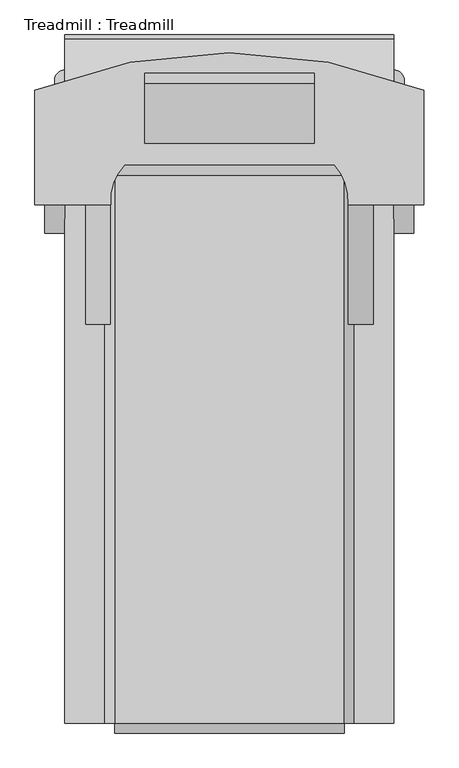
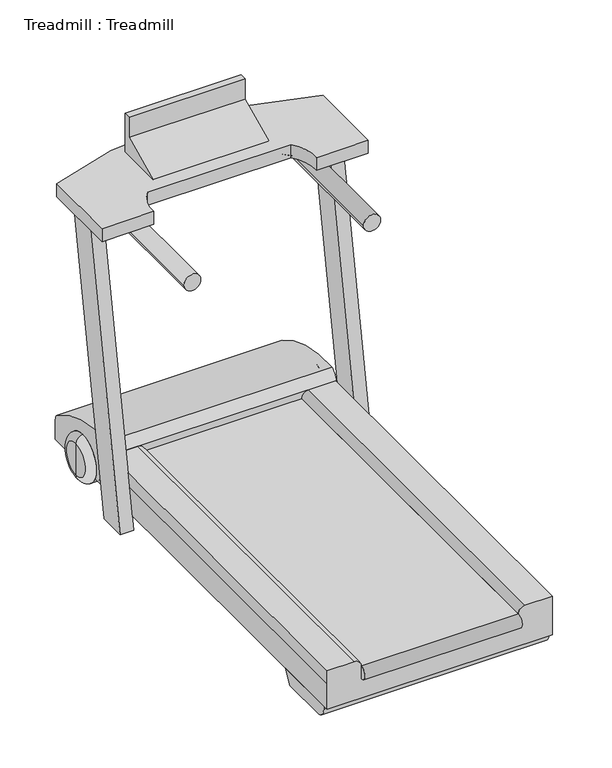
"""IFC4 building model written with IfcOpenShell, lengths in millimetres: proxy geometry, Treadmill : Treadmill."""

from ifc_helpers import new_model, si_unit, point, frame, frame_2d, origin, place, context, project, spatial, polyline, circle_curve, ellipse_curve, trimmed, segment, composite_curve, outline, extrude, source, transform, mapped, element, save
from ifc_brep_helpers import plane_surface, cylinder_surface, revolved_surface, advanced_brep


def treadmill_treadmill_b3c1e061(model_context):
    return source(origin(), model_context, "Body", "SolidModel", [
        extrude(outline(composite_curve([segment(polyline([(152.4, 152.4), (177.8, 152.4)]), True, "CONTINUOUS"), segment(trimmed(circle_curve(frame_2d((177.8, 127.0)), 25.4), [point((177.8, 152.4))], [point((203.2, 127.0))], False, "CARTESIAN"), True, "CONTINUOUS"), segment(polyline([(203.2, 127.0), (203.2, 25.4), (152.4, 25.4), (50.8, 25.4), (50.8, 863.6), (152.4, 863.6), (203.2, 863.6), (203.2, 762.0)]), True, "CONTINUOUS"), segment(trimmed(circle_curve(frame_2d((177.8, 762.0)), 25.4), [point((203.2, 762.0))], [point((177.8, 736.6))], False, "CARTESIAN"), True, "CONTINUOUS"), segment(polyline([(177.8, 736.6), (152.4, 736.6), (152.4, 152.4)]), True, "CONTINUOUS")], self_intersect=False)), frame((0.0, -1752.6, 0.0), z_axis=(0.0, 1.0, 0.0), x_axis=(0.0, 0.0, 1.0)), (0.0, 0.0, 1.0), 1397.0),
        extrude(outline(composite_curve([segment(polyline([(-356.6198638, 50.8), (-356.6198638, 204.4296136)]), True, "CONTINUOUS"), segment(trimmed(circle_curve(frame_2d((-319.002006, 205.4588927)), 37.6319364), [point((-356.6198638, 204.4296136))], [point((-330.6373426, 241.2469016))], False, "CARTESIAN"), True, "CONTINUOUS"), segment(trimmed(circle_curve(frame_2d((-289.1455701, -230.6771793)), 473.744557), [point((-330.6373426, 241.2469016))], [point((-10.4238809, 152.4))], False, "CARTESIAN"), True, "CONTINUOUS"), segment(trimmed(circle_curve(frame_2d((-36.1581881, 127.0)), 36.1581881), [point((-10.4238809, 152.4))], [point((0.0, 127.0))], False, "CARTESIAN"), True, "CONTINUOUS"), segment(polyline([(0.0, 127.0), (0.0, 50.8), (-356.6198638, 50.8)]), True, "CONTINUOUS")], self_intersect=False)), frame((25.4, 0.0, 0.0), z_axis=(1.0, 0.0, 0.0), x_axis=(0.0, 1.0, 0.0)), (0.0, 0.0, 1.0), 838.2),
        extrude(outline(composite_curve([segment(polyline([(-355.6, 152.4), (-1752.6, 152.4), (-1752.6, 127.0)]), True, "CONTINUOUS"), segment(trimmed(circle_curve(frame_2d((-1752.6, 152.4)), 25.4), [point((-1752.6, 127.0))], [point((-1752.6, 177.8))], False, "CARTESIAN"), True, "CONTINUOUS"), segment(polyline([(-1752.6, 177.8), (-355.6, 177.8), (-355.6, 152.4)]), True, "CONTINUOUS")], self_intersect=False)), frame((152.4, 0.0, 0.0), z_axis=(1.0, 0.0, 0.0), x_axis=(0.0, 1.0, 0.0)), (0.0, 0.0, 1.0), 584.2),
        advanced_brep(
        [(25.3285406, -177.8, 177.8), (50.8, -177.8, 177.8), (50.8, -177.8, 0.0), (25.3285406, -177.8, 0.0), (-0.7314789, -177.8, 151.7399805), (-0.7314789, -177.8, 26.0600195), (-0.7314789, -177.8, 88.9), (50.8, -177.8, 88.9)],
        [
            (0, 1),
            (1, 2, circle_curve(frame((50.8, -177.8, 88.9), z_axis=(-1.0, 0.0, 0.0), x_axis=(0.0, 0.0, -1.0)), 88.9)),
            (2, 3),
            (3, 0, circle_curve(frame((25.3285406, -177.8, 88.9), z_axis=(1.0, 0.0, 0.0), x_axis=(0.0, 0.0, -1.0)), 88.9)),
            (2, 1, circle_curve(frame((50.8, -177.8, 88.9), z_axis=(-1.0, 0.0, 0.0), x_axis=(0.0, 0.0, -1.0)), 88.9)),
            (0, 3, circle_curve(frame((25.3285406, -177.8, 88.9), z_axis=(1.0, 0.0, 0.0), x_axis=(0.0, 0.0, -1.0)), 88.9)),
            (4, 0, circle_curve(frame((25.3285406, -177.8, 151.7399805), z_axis=(0.0, 1.0, 0.0), x_axis=(0.0, 0.0, 1.0)), 26.0600195)),
            (3, 5, circle_curve(frame((25.3285406, -177.8, 26.0600195), z_axis=(0.0, 1.0, 0.0), x_axis=(0.0, 0.0, -1.0)), 26.0600195)),
            (5, 4, circle_curve(frame((-0.7314789, -177.8, 88.9), z_axis=(1.0, 0.0, 0.0), x_axis=(0.0, 0.0, -1.0)), 62.8399805)),
            (4, 5, circle_curve(frame((-0.7314789, -177.8, 88.9), z_axis=(1.0, 0.0, 0.0), x_axis=(0.0, 0.0, -1.0)), 62.8399805)),
            (6, 4),
            (5, 6),
            (1, 7),
            (7, 2),
        ],
        [
            cylinder_surface(frame((-0.7314789, -177.8, 88.9), z_axis=(-1.0, 0.0, 0.0), x_axis=(0.0, 0.0, -1.0)), 88.9),
            revolved_surface(trimmed(ellipse_curve(frame((25.3285406, -177.8, 26.0600195), z_axis=(0.0, 1.0, 0.0), x_axis=(0.0, 0.0, -1.0)), 26.0600195, 26.0600195), [point((25.3285406, -177.8, 0.0))], [point((-0.7314789, -177.8, 26.0600195))], True, "CARTESIAN"), (-0.7314789, -177.8, 88.9), (-1.0, 0.0, 0.0)),
            plane_surface(frame((-0.7314789, -177.8, 88.9), z_axis=(-1.0, 0.0, 0.0), x_axis=(0.0, 0.0, -1.0))),
            plane_surface(frame((50.8, -177.8, 88.9), z_axis=(1.0, 0.0, 0.0), x_axis=(0.0, 0.0, -1.0))),
        ],
        [
            (0, [[1, 2, 3, 4]]),
            (0, [[-3, 5, -1, 6]]),
            (1, [[7, -4, 8, 9]]),
            (1, [[-8, -6, -7, 10]]),
            (2, [[11, -9, 12]]),
            (2, [[-12, -10, -11]]),
            (3, [[13, 14, -2]]),
            (3, [[-14, -13, -5]]),
        ],
    ),
        advanced_brep(
        [(838.2, -177.8, 88.9), (838.2, -177.8, 177.8), (838.2, -177.8, 0.0), (889.7314789, -177.8, 151.7399805), (889.7314789, -177.8, 88.9), (889.7314789, -177.8, 26.0600195), (863.6714594, -177.8, 177.8), (863.6714594, -177.8, 0.0)],
        [
            (0, 1),
            (1, 2, circle_curve(frame((838.2, -177.8, 88.9), z_axis=(-1.0, 0.0, 0.0), x_axis=(0.0, 0.0, -1.0)), 88.9)),
            (2, 0),
            (2, 1, circle_curve(frame((838.2, -177.8, 88.9), z_axis=(-1.0, 0.0, 0.0), x_axis=(0.0, 0.0, -1.0)), 88.9)),
            (3, 4),
            (4, 5),
            (5, 3, circle_curve(frame((889.7314789, -177.8, 88.9), z_axis=(1.0, 0.0, 0.0), x_axis=(0.0, 0.0, -1.0)), 62.8399805)),
            (3, 5, circle_curve(frame((889.7314789, -177.8, 88.9), z_axis=(1.0, 0.0, 0.0), x_axis=(0.0, 0.0, -1.0)), 62.8399805)),
            (6, 3, circle_curve(frame((863.6714594, -177.8, 151.7399805), z_axis=(0.0, 1.0, 0.0), x_axis=(0.0, 0.0, 1.0)), 26.0600195)),
            (5, 7, circle_curve(frame((863.6714594, -177.8, 26.0600195), z_axis=(0.0, 1.0, 0.0), x_axis=(0.0, 0.0, -1.0)), 26.0600195)),
            (7, 6, circle_curve(frame((863.6714594, -177.8, 88.9), z_axis=(1.0, 0.0, 0.0), x_axis=(0.0, 0.0, -1.0)), 88.9)),
            (6, 7, circle_curve(frame((863.6714594, -177.8, 88.9), z_axis=(1.0, 0.0, 0.0), x_axis=(0.0, 0.0, -1.0)), 88.9)),
            (1, 6),
            (7, 2),
        ],
        [
            plane_surface(frame((838.2, -177.8, 88.9), z_axis=(-1.0, 0.0, 0.0), x_axis=(0.0, 0.0, -1.0))),
            plane_surface(frame((889.7314789, -177.8, 88.9), z_axis=(1.0, 0.0, 0.0), x_axis=(0.0, 0.0, -1.0))),
            revolved_surface(trimmed(ellipse_curve(frame((863.6714594, -177.8, 26.0600195), z_axis=(0.0, 1.0, 0.0), x_axis=(0.0, 0.0, -1.0)), 26.0600195, 26.0600195), [point((889.7314789, -177.8, 26.0600195))], [point((863.6714594, -177.8, 0.0))], True, "CARTESIAN"), (889.7314789, -177.8, 88.9), (-1.0, 0.0, 0.0)),
            cylinder_surface(frame((889.7314789, -177.8, 88.9), z_axis=(-1.0, 0.0, 0.0), x_axis=(0.0, 0.0, -1.0)), 88.9),
        ],
        [
            (0, [[1, 2, 3]]),
            (0, [[-3, 4, -1]]),
            (1, [[5, 6, 7]]),
            (1, [[-6, -5, 8]]),
            (2, [[9, -7, 10, 11]]),
            (2, [[-10, -8, -9, 12]]),
            (3, [[13, -11, 14, -2]]),
            (3, [[-14, -12, -13, -4]]),
        ],
    ),
        extrude(outline(composite_curve([segment(polyline([(-1514.6655035, 0.0), (-1693.1449893, 0.0)]), True, "CONTINUOUS"), segment(trimmed(circle_curve(frame_2d((-1693.1449893, 38.1)), 38.1), [point((-1693.1449893, 0.0))], [point((-1731.2449893, 38.1))], False, "CARTESIAN"), True, "CONTINUOUS"), segment(polyline([(-1731.2449893, 38.1), (-1731.2449893, 50.8), (-1483.7010673, 50.8), (-1514.6655035, 0.0)]), True, "CONTINUOUS")], self_intersect=False)), frame((25.4, 0.0, 0.0), z_axis=(1.0, 0.0, 0.0), x_axis=(0.0, 1.0, 0.0)), (0.0, 0.0, 1.0), 838.2),
        extrude(outline(polyline([(-204.732057, 1117.6), (-401.7950906, 0.0), (-504.9624344, 0.0), (-307.8994008, 1117.6), (-204.732057, 1117.6)])), frame((863.6, 0.0, 0.0), z_axis=(1.0, 0.0, 0.0), x_axis=(0.0, 1.0, 0.0)), (0.0, 0.0, 1.0), 50.8),
        extrude(outline(polyline([(-204.732057, 1117.6), (-401.7950906, 0.0), (-504.9624344, 0.0), (-307.8994008, 1117.6), (-204.732057, 1117.6)])), frame((-25.4, 0.0, 0.0), z_axis=(1.0, 0.0, 0.0), x_axis=(0.0, 1.0, 0.0)), (0.0, 0.0, 1.0), 50.8),
        extrude(outline(composite_curve([segment(trimmed(circle_curve(frame_2d((444.5, -1366.4086936)), 1321.3993645), [point((-50.8, -141.347801))], [point((939.8, -141.347801))], False, "CARTESIAN"), True, "CONTINUOUS"), segment(polyline([(939.8, -141.347801), (939.8, -432.8198638), (746.8275156, -432.8198638)]), True, "CONTINUOUS"), segment(trimmed(circle_curve(frame_2d((612.8803133, -422.2461786)), 134.3638933), [point((746.8275156, -432.8198638))], [point((711.1731257, -330.6373426))], True, "CARTESIAN"), True, "CONTINUOUS"), segment(polyline([(711.1731257, -330.6373426), (177.8268743, -330.6373426)]), True, "CONTINUOUS"), segment(trimmed(circle_curve(frame_2d((276.1196867, -422.2461786)), 134.3638933), [point((177.8268743, -330.6373426))], [point((142.1724844, -432.8198638))], True, "CARTESIAN"), True, "CONTINUOUS"), segment(polyline([(142.1724844, -432.8198638), (-50.8, -432.8198638), (-50.8, -141.347801)]), True, "CONTINUOUS")], self_intersect=False)), frame((0.0, 0.0, 1117.6), z_axis=(0.0, 0.0, 1.0), x_axis=(1.0, 0.0, 0.0)), (0.0, 0.0, 1.0), 50.8),
        advanced_brep(
        [(78.1863004, -736.6, 1085.0214532), (141.6863004, -736.6, 1085.0214532), (141.6863004, -255.3253298, 1085.0214532), (78.1863004, -229.0227686, 1085.0214532), (154.6909766, -242.3206537, 1085.0214532), (128.3884153, -178.8206537, 1085.0214532), (734.3090234, -242.3206537, 1085.0214532), (760.6115847, -178.8206537, 1085.0214532), (747.3136996, -255.3253298, 1085.0214532), (810.8136996, -229.0227686, 1085.0214532), (810.8136996, -736.6, 1085.0214532), (747.3136996, -736.6, 1085.0214532)],
        [
            (0, 1, circle_curve(frame((109.9363004, -736.6, 1085.0214532), z_axis=(0.0, -1.0, 0.0), x_axis=(1.0, 0.0, 0.0)), 31.75)),
            (1, 0, circle_curve(frame((109.9363004, -736.6, 1085.0214532), z_axis=(0.0, -1.0, 0.0), x_axis=(1.0, 0.0, 0.0)), 31.75)),
            (1, 2),
            (2, 3, ellipse_curve(frame((109.9363004, -242.1740492, 1085.0214532), z_axis=(-0.382683432365089, -0.9238795325112871, 0.0), x_axis=(0.9238795325112872, -0.3826834323650889, 0.0)), 34.3659524, 31.75)),
            (3, 0),
            (3, 2, ellipse_curve(frame((109.9363004, -242.1740492, 1085.0214532), z_axis=(-0.382683432365089, -0.9238795325112871, 0.0), x_axis=(0.9238795325112872, -0.3826834323650889, 0.0)), 34.3659524, 31.75)),
            (2, 4),
            (4, 5, ellipse_curve(frame((141.5396959, -210.5706537, 1085.0214532), z_axis=(-0.9238795325112865, -0.3826834323650906, 0.0), x_axis=(0.38268343236509084, -0.9238795325112864, 0.0)), 34.3659524, 31.75)),
            (5, 3),
            (5, 4, ellipse_curve(frame((141.5396959, -210.5706537, 1085.0214532), z_axis=(-0.9238795325112865, -0.3826834323650906, 0.0), x_axis=(0.38268343236509084, -0.9238795325112864, 0.0)), 34.3659524, 31.75)),
            (4, 6),
            (6, 7, ellipse_curve(frame((747.4603041, -210.5706537, 1085.0214532), z_axis=(-0.9238795325112865, 0.3826834323650905, 0.0), x_axis=(-0.38268343236509034, -0.9238795325112866, 0.0)), 34.3659524, 31.75)),
            (7, 5),
            (7, 6, ellipse_curve(frame((747.4603041, -210.5706537, 1085.0214532), z_axis=(-0.9238795325112865, 0.3826834323650905, 0.0), x_axis=(-0.38268343236509034, -0.9238795325112866, 0.0)), 34.3659524, 31.75)),
            (6, 8),
            (8, 9, ellipse_curve(frame((779.0636996, -242.1740492, 1085.0214532), z_axis=(-0.382683432365089, 0.923879532511287, 0.0), x_axis=(-0.9238795325112873, -0.38268343236508884, 0.0)), 34.3659524, 31.75)),
            (9, 7),
            (9, 8, ellipse_curve(frame((779.0636996, -242.1740492, 1085.0214532), z_axis=(-0.382683432365089, 0.923879532511287, 0.0), x_axis=(-0.9238795325112873, -0.38268343236508884, 0.0)), 34.3659524, 31.75)),
            (10, 11, circle_curve(frame((779.0636996, -736.6, 1085.0214532), z_axis=(0.0, -1.0, 0.0), x_axis=(-1.0, 0.0, 0.0)), 31.75)),
            (11, 10, circle_curve(frame((779.0636996, -736.6, 1085.0214532), z_axis=(0.0, -1.0, 0.0), x_axis=(-1.0, 0.0, 0.0)), 31.75)),
            (8, 11),
            (10, 9),
        ],
        [
            plane_surface(frame((-1038.8645002, -736.6, 0.0), z_axis=(0.0, -1.0, 0.0), x_axis=(0.0, 0.0, -1.0))),
            cylinder_surface(frame((109.9363004, -736.6, 1085.0214532), z_axis=(0.0, -1.0, 0.0), x_axis=(1.0, 0.0, 0.0)), 31.75),
            cylinder_surface(frame((100.3379982, -251.7723515, 1085.0214532), z_axis=(-0.7071067811865464, -0.7071067811865488, 0.0), x_axis=(0.7071067811865488, -0.7071067811865464, 0.0)), 31.75),
            cylinder_surface(frame((127.9656467, -210.5706537, 1085.0214532), z_axis=(-1.0, 0.0, 0.0), x_axis=(0.0, -1.0, 0.0)), 31.75),
            cylinder_surface(frame((737.8620018, -200.9723515, 1085.0214532), z_axis=(-0.7071067811865465, 0.7071067811865487, 0.0), x_axis=(-0.7071067811865487, -0.7071067811865465, 0.0)), 31.75),
            plane_surface(frame((-304.1957937, -736.6, 0.0), z_axis=(0.0, -1.0, 0.0), x_axis=(0.0, 0.0, 1.0))),
            cylinder_surface(frame((779.0636996, -228.6, 1085.0214532), z_axis=(0.0, 1.0, 0.0), x_axis=(-1.0, 0.0, 0.0)), 31.75),
        ],
        [
            (0, [[1, 2]]),
            (1, [[3, 4, 5, -2]]),
            (1, [[-5, 6, -3, -1]]),
            (2, [[7, 8, 9, -4]]),
            (2, [[-9, 10, -7, -6]]),
            (3, [[11, 12, 13, -8]]),
            (3, [[-13, 14, -11, -10]]),
            (4, [[15, 16, 17, -12]]),
            (4, [[-17, 18, -15, -14]]),
            (5, [[19, 20]]),
            (6, [[21, -19, 22, -16]]),
            (6, [[-22, -20, -21, -18]]),
        ],
    ),
        extrude(outline(polyline([(-122.6746955, 1240.8350591), (-122.6746955, 1320.8), (-97.2746955, 1320.8), (-97.2746955, 1231.9), (-97.2746955, 1168.4), (-277.1099218, 1168.4), (-122.6746955, 1240.8350591)])), frame((228.6, 0.0, 0.0), z_axis=(1.0, 0.0, 0.0), x_axis=(0.0, 1.0, 0.0)), (0.0, 0.0, 1.0), 431.8),
    ])


if __name__ == "__main__":
    model = new_model("IFC4")
    model_context = context("Model", 3, world=origin())
    ifc_project = project(units=[si_unit("LENGTHUNIT", "METRE", prefix="MILLI")], contexts=[model_context])
    site = spatial("IfcSite", under=ifc_project)
    building = spatial("IfcBuilding", under=site)
    placement = place(None, origin())
    treadmill_treadmill_shape = treadmill_treadmill_b3c1e061(model_context)
    element("IfcBuildingElementProxy", 1, Name="Treadmill : Treadmill", ObjectType="Treadmill : Treadmill", at=placement, inside=building, context=model_context, shape_type="MappedRepresentation", body=[
        mapped(treadmill_treadmill_shape, transform((0.0, 0.0, 0.0), x_axis=(1.0, 0.0, 0.0), y_axis=(0.0, 1.0, 0.0), z_axis=(0.0, 0.0, 1.0))),
    ])
    save(model, "model.ifc")

# Revit data of these elements
# Type "Treadmill : Treadmill"
#   Assembly Code = "E1090"
#   Default Elevation = 0
# Element 1 (IfcBuildingElementProxy, "Treadmill : Treadmill")
#   Materials on its faces: "Metal - Steel"
# Materials
#   "Metal - Steel": colour RGB 210 210 210, transparency 0
